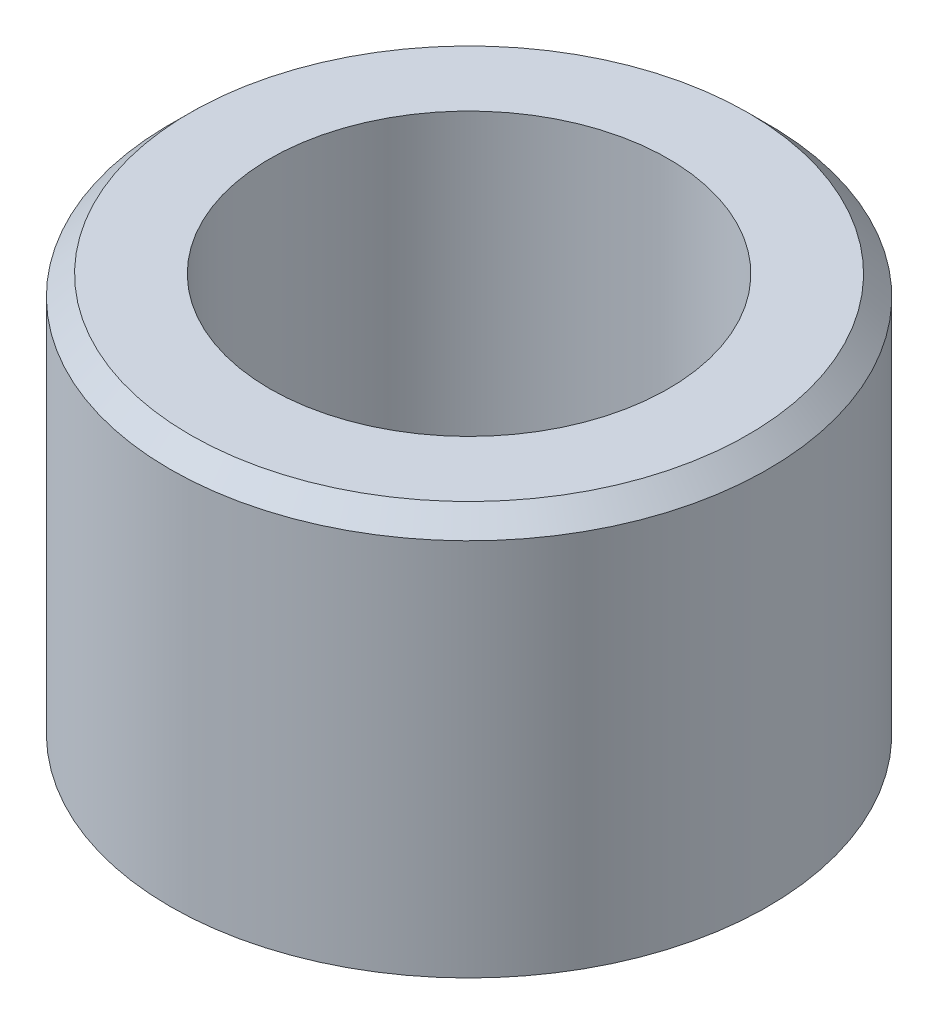
SolidWorks part; units mm, degrees
material "Plain Carbon Steel"
ref_plane "Front Plane" through (0, 0, 0) normal (0, 0, 1) x (1, 0, 0)
ref_plane "Top Plane" through (0, 0, 0) normal (0, 1, 0) x (1, 0, 0)
ref_plane "Right Plane" through (0, 0, 0) normal (1, 0, 0) x (0, 0, -1)
sketch "Bush Profile Ø30-Ø20" plane through (0, 0, 0) normal (0, 1, 0) x (1, 0, 0)
  circle A0 centre (0, 0) radius 15
  circle A1 centre (0, 0) radius 10
  dimension "D1" = 30
  dimension "D2" = 20
extrude "Bush Body L20" add sketch "Bush Profile Ø30-Ø20" along normal blind 20
chamfer "Outer Edge Chamfer 1x45°" distance 1 angle 45 1 edges at (0, 20, 15)
